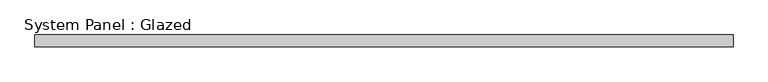
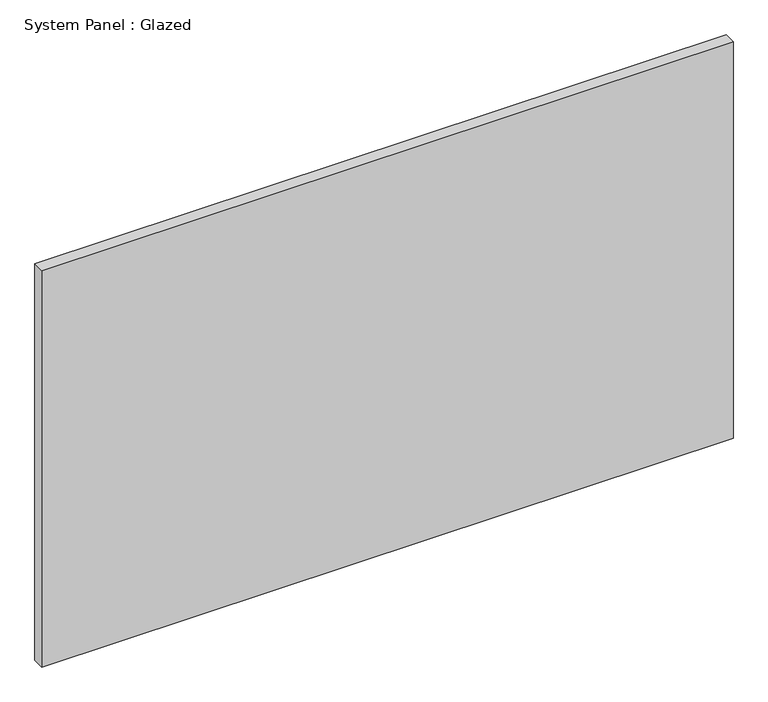
"""IFC4 building model written with IfcOpenShell, lengths in millimetres: plate geometry, System Panel : Glazed."""

from ifc_helpers import new_model, si_unit, origin, origin_with_axes, place, context, project, spatial, polyline, outline, extrude, source, transform, mapped, element, save


def system_panel_glazed_4be86f7f(model_context):
    return source(origin(), model_context, "Body", "SweptSolid", [
        extrude(outline(polyline([(754.1325975, 19.05), (-754.1325975, 19.05), (-754.1325975, 44.45), (754.1325975, 44.45), (754.1325975, 19.05)])), origin_with_axes(), (0.0, 0.0, 1.0), 914.4),
    ])


if __name__ == "__main__":
    model = new_model("IFC4")
    model_context = context("Model", 3, world=origin())
    ifc_project = project(units=[si_unit("LENGTHUNIT", "METRE", prefix="MILLI")], contexts=[model_context])
    site = spatial("IfcSite", under=ifc_project)
    building = spatial("IfcBuilding", under=site)
    placement = place(None, origin())
    system_panel_glazed_shape = system_panel_glazed_4be86f7f(model_context)
    element("IfcPlate", 1, ObjectType="System Panel : Glazed", at=placement, inside=building, context=model_context, shape_type="MappedRepresentation", body=[
        mapped(system_panel_glazed_shape, transform((0.0, 0.0, 0.0), x_axis=(1.0, 0.0, 0.0), y_axis=(0.0, 1.0, 0.0), z_axis=(0.0, 0.0, 1.0))),
    ])
    save(model, "model.ifc")

# Revit data of these elements
# Type "System Panel : Glazed"
#   Construction Type Id = "GSP4R"
#   Analytic Construction = "1/8 in Pilkington single glazing"
#   Visual Light Transmittance = 0.9
#   Solar Heat Gain Coefficient = 0.86
#   Heat Transfer Coefficient (U) = 6.7069 W/(m²·K)
# Element 1 (IfcPlate, "System Panel : Glazed")
#   Materials on its faces: "Glass"
# Materials
#   "Glass": class "Glass", colour RGB 0 128 192, transparency 0.75, Description = "Soda Lime Glass", Cost = 0
